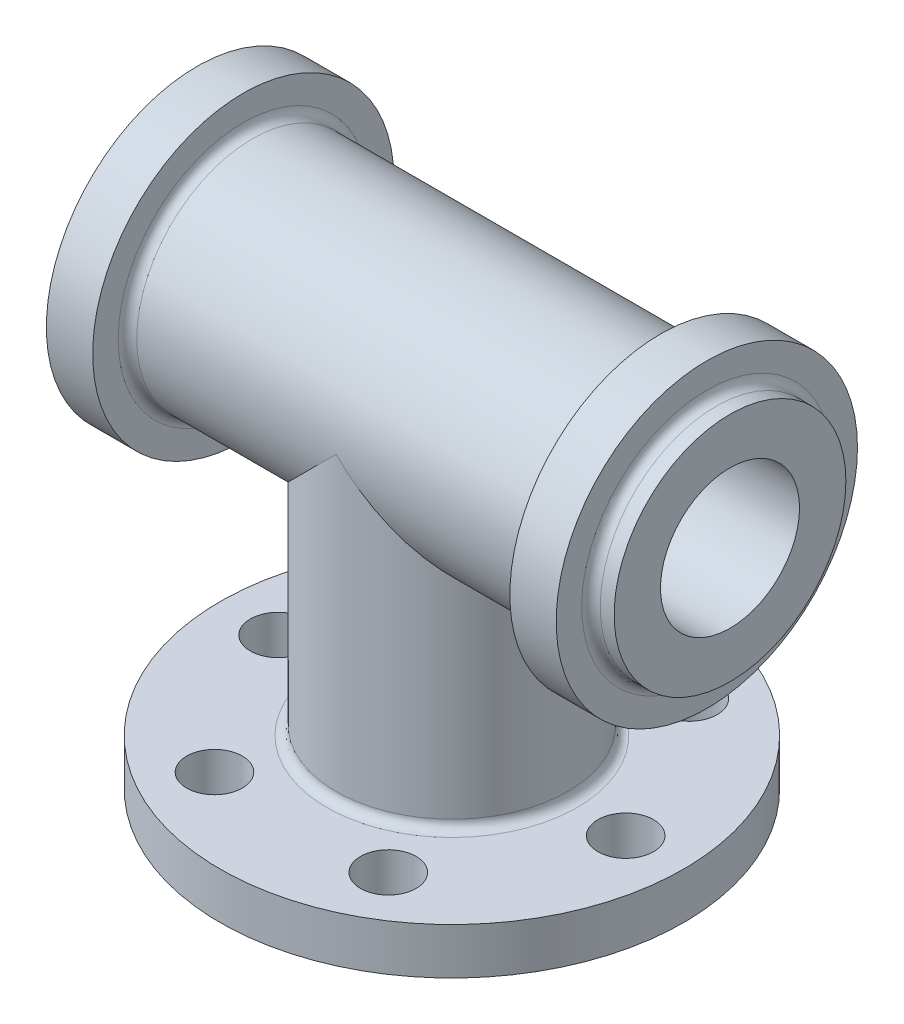
ISO-10303-21;
HEADER;
FILE_DESCRIPTION(('STEP AP214'),'2;1');
FILE_NAME('part.step','',(''),(''),'','','');
FILE_SCHEMA(('AUTOMOTIVE_DESIGN { 1 0 10303 214 1 1 1 1 }'));
ENDSEC;
DATA;
#1=APPLICATION_CONTEXT('core data for automotive mechanical design processes');
#2=APPLICATION_PROTOCOL_DEFINITION('international standard','automotive_design',2000,#1);
#3=PRODUCT_CONTEXT('',#1,'mechanical');
#4=PRODUCT('Part','Part','',(#3));
#5=PRODUCT_RELATED_PRODUCT_CATEGORY('part','',(#4));
#6=PRODUCT_DEFINITION_FORMATION('','',#4);
#7=PRODUCT_DEFINITION_CONTEXT('part definition',#1,'design');
#8=PRODUCT_DEFINITION('design','',#6,#7);
#9=PRODUCT_DEFINITION_SHAPE('','',#8);
#10=(LENGTH_UNIT() NAMED_UNIT(*) SI_UNIT(.MILLI.,.METRE.));
#11=(NAMED_UNIT(*) PLANE_ANGLE_UNIT() SI_UNIT($,.RADIAN.));
#12=(NAMED_UNIT(*) SI_UNIT($,.STERADIAN.) SOLID_ANGLE_UNIT());
#13=UNCERTAINTY_MEASURE_WITH_UNIT(LENGTH_MEASURE(1.E-05),#10,'distance_accuracy_value','');
#14=(GEOMETRIC_REPRESENTATION_CONTEXT(3) GLOBAL_UNCERTAINTY_ASSIGNED_CONTEXT((#13)) GLOBAL_UNIT_ASSIGNED_CONTEXT((#10,
#11,#12)) REPRESENTATION_CONTEXT('',''));
#15=CARTESIAN_POINT('',(0.,0.,0.));
#16=DIRECTION('',(0.,0.,1.));
#17=DIRECTION('',(1.,0.,0.));
#18=AXIS2_PLACEMENT_3D('',#15,#16,#17);
#19=CARTESIAN_POINT('',(0.,-80.,0.));
#20=DIRECTION('',(0.,1.,0.));
#21=DIRECTION('',(0.,0.,1.));
#22=AXIS2_PLACEMENT_3D('',#19,#20,#21);
#23=CYLINDRICAL_SURFACE('',#22,25.);
#24=CARTESIAN_POINT('',(0.,-63.,0.));
#25=DIRECTION('',(0.,-1.,0.));
#26=DIRECTION('',(0.,0.,-1.));
#27=AXIS2_PLACEMENT_3D('',#24,#25,#26);
#28=CIRCLE('',#27,25.);
#29=CARTESIAN_POINT('',(0.,-63.,-25.));
#30=VERTEX_POINT('',#29);
#31=EDGE_CURVE('E81',#30,#30,#28,.F.);
#32=ORIENTED_EDGE('',*,*,#31,.T.);
#33=EDGE_LOOP('',(#32));
#34=FACE_BOUND('',#33,.T.);
#35=CARTESIAN_POINT('',(0.,0.,0.));
#36=DIRECTION('',(-0.707106781186547,0.707106781186547,0.));
#37=DIRECTION('',(-0.707106781186547,-0.707106781186547,0.));
#38=AXIS2_PLACEMENT_3D('',#35,#36,#37);
#39=ELLIPSE('',#38,35.3553390593274,25.);
#40=CARTESIAN_POINT('',(0.,0.,-25.));
#41=VERTEX_POINT('',#40);
#42=CARTESIAN_POINT('',(0.,0.,25.));
#43=VERTEX_POINT('',#42);
#44=EDGE_CURVE('E65',#41,#43,#39,.T.);
#45=ORIENTED_EDGE('',*,*,#44,.F.);
#46=CARTESIAN_POINT('',(0.,0.,0.));
#47=DIRECTION('',(-0.707106781186547,-0.707106781186547,0.));
#48=DIRECTION('',(-0.707106781186547,0.707106781186547,0.));
#49=AXIS2_PLACEMENT_3D('',#46,#47,#48);
#50=ELLIPSE('',#49,35.3553390593274,25.);
#51=EDGE_CURVE('E182',#43,#41,#50,.F.);
#52=ORIENTED_EDGE('',*,*,#51,.F.);
#53=EDGE_LOOP('',(#45,#52));
#54=FACE_BOUND('',#53,.T.);
#55=ADVANCED_FACE('F41',(#34,#54),#23,.T.);
#56=CARTESIAN_POINT('',(60.,0.,0.));
#57=DIRECTION('',(-1.,0.,0.));
#58=DIRECTION('',(0.,0.,1.));
#59=AXIS2_PLACEMENT_3D('',#56,#57,#58);
#60=CYLINDRICAL_SURFACE('',#59,25.);
#61=CARTESIAN_POINT('',(43.,0.,0.));
#62=DIRECTION('',(1.,0.,0.));
#63=DIRECTION('',(0.,0.,-1.));
#64=AXIS2_PLACEMENT_3D('',#61,#62,#63);
#65=CIRCLE('',#64,25.);
#66=CARTESIAN_POINT('',(43.,0.,-25.));
#67=VERTEX_POINT('',#66);
#68=EDGE_CURVE('E98',#67,#67,#65,.F.);
#69=ORIENTED_EDGE('',*,*,#68,.T.);
#70=EDGE_LOOP('',(#69));
#71=FACE_BOUND('',#70,.T.);
#72=CARTESIAN_POINT('',(-43.,0.,0.));
#73=DIRECTION('',(-1.,0.,0.));
#74=DIRECTION('',(0.,0.,1.));
#75=AXIS2_PLACEMENT_3D('',#72,#73,#74);
#76=CIRCLE('',#75,25.);
#77=CARTESIAN_POINT('',(-43.,0.,25.));
#78=VERTEX_POINT('',#77);
#79=EDGE_CURVE('E92',#78,#78,#76,.F.);
#80=ORIENTED_EDGE('',*,*,#79,.T.);
#81=EDGE_LOOP('',(#80));
#82=FACE_BOUND('',#81,.T.);
#83=ORIENTED_EDGE('',*,*,#51,.T.);
#84=ORIENTED_EDGE('',*,*,#44,.T.);
#85=EDGE_LOOP('',(#83,#84));
#86=FACE_BOUND('',#85,.T.);
#87=ADVANCED_FACE('F127',(#71,#82,#86),#60,.T.);
#88=CARTESIAN_POINT('',(45.,0.,0.));
#89=DIRECTION('',(1.,0.,0.));
#90=DIRECTION('',(0.,0.,-1.));
#91=AXIS2_PLACEMENT_3D('',#88,#89,#90);
#92=CYLINDRICAL_SURFACE('',#91,32.5);
#93=CARTESIAN_POINT('',(45.,0.,0.));
#94=DIRECTION('',(1.,0.,0.));
#95=DIRECTION('',(0.,0.,-1.));
#96=AXIS2_PLACEMENT_3D('',#93,#94,#95);
#97=CIRCLE('',#96,32.5);
#98=CARTESIAN_POINT('',(45.,0.,-32.5));
#99=VERTEX_POINT('',#98);
#100=EDGE_CURVE('E174',#99,#99,#97,.T.);
#101=ORIENTED_EDGE('',*,*,#100,.T.);
#102=EDGE_LOOP('',(#101));
#103=FACE_BOUND('',#102,.T.);
#104=CARTESIAN_POINT('',(55.,0.,0.));
#105=DIRECTION('',(1.,0.,0.));
#106=DIRECTION('',(0.,0.,-1.));
#107=AXIS2_PLACEMENT_3D('',#104,#105,#106);
#108=CIRCLE('',#107,32.5);
#109=CARTESIAN_POINT('',(55.,0.,-32.5));
#110=VERTEX_POINT('',#109);
#111=EDGE_CURVE('E168',#110,#110,#108,.T.);
#112=ORIENTED_EDGE('',*,*,#111,.F.);
#113=EDGE_LOOP('',(#112));
#114=FACE_BOUND('',#113,.T.);
#115=ADVANCED_FACE('F131',(#103,#114),#92,.T.);
#116=CARTESIAN_POINT('',(45.,0.,0.));
#117=DIRECTION('',(1.,0.,0.));
#118=DIRECTION('',(0.,0.,-1.));
#119=AXIS2_PLACEMENT_3D('',#116,#117,#118);
#120=PLANE('',#119);
#121=CARTESIAN_POINT('',(45.,0.,0.));
#122=DIRECTION('',(1.,0.,0.));
#123=DIRECTION('',(0.,0.,-1.));
#124=AXIS2_PLACEMENT_3D('',#121,#122,#123);
#125=CIRCLE('',#124,27.);
#126=CARTESIAN_POINT('',(45.,0.,-27.));
#127=VERTEX_POINT('',#126);
#128=EDGE_CURVE('E95',#127,#127,#125,.T.);
#129=ORIENTED_EDGE('',*,*,#128,.T.);
#130=EDGE_LOOP('',(#129));
#131=FACE_BOUND('',#130,.T.);
#132=ORIENTED_EDGE('',*,*,#100,.F.);
#133=EDGE_LOOP('',(#132));
#134=FACE_BOUND('',#133,.T.);
#135=ADVANCED_FACE('F239',(#131,#134),#120,.F.);
#136=CARTESIAN_POINT('',(55.,0.,0.));
#137=DIRECTION('',(1.,0.,0.));
#138=DIRECTION('',(0.,0.,-1.));
#139=AXIS2_PLACEMENT_3D('',#136,#137,#138);
#140=PLANE('',#139);
#141=CARTESIAN_POINT('',(55.,0.,0.));
#142=DIRECTION('',(1.,0.,0.));
#143=DIRECTION('',(0.,0.,-1.));
#144=AXIS2_PLACEMENT_3D('',#141,#142,#143);
#145=CIRCLE('',#144,27.);
#146=CARTESIAN_POINT('',(55.,0.,-27.));
#147=VERTEX_POINT('',#146);
#148=EDGE_CURVE('E90',#147,#147,#145,.F.);
#149=ORIENTED_EDGE('',*,*,#148,.T.);
#150=EDGE_LOOP('',(#149));
#151=FACE_BOUND('',#150,.T.);
#152=ORIENTED_EDGE('',*,*,#111,.T.);
#153=EDGE_LOOP('',(#152));
#154=FACE_BOUND('',#153,.T.);
#155=ADVANCED_FACE('F244',(#151,#154),#140,.T.);
#156=CARTESIAN_POINT('',(60.,0.,0.));
#157=DIRECTION('',(1.,0.,0.));
#158=DIRECTION('',(0.,0.,-1.));
#159=AXIS2_PLACEMENT_3D('',#156,#157,#158);
#160=PLANE('',#159);
#161=CARTESIAN_POINT('',(60.,0.,0.));
#162=DIRECTION('',(1.,0.,0.));
#163=DIRECTION('',(0.,0.,-1.));
#164=AXIS2_PLACEMENT_3D('',#161,#162,#163);
#165=CIRCLE('',#164,15.);
#166=CARTESIAN_POINT('',(60.,0.,-15.));
#167=VERTEX_POINT('',#166);
#168=EDGE_CURVE('E164',#167,#167,#165,.T.);
#169=ORIENTED_EDGE('',*,*,#168,.F.);
#170=EDGE_LOOP('',(#169));
#171=FACE_BOUND('',#170,.T.);
#172=CARTESIAN_POINT('',(60.,0.,0.));
#173=DIRECTION('',(1.,0.,0.));
#174=DIRECTION('',(0.,0.,-1.));
#175=AXIS2_PLACEMENT_3D('',#172,#173,#174);
#176=CIRCLE('',#175,25.);
#177=CARTESIAN_POINT('',(60.,0.,-25.));
#178=VERTEX_POINT('',#177);
#179=EDGE_CURVE('E176',#178,#178,#176,.T.);
#180=ORIENTED_EDGE('',*,*,#179,.T.);
#181=EDGE_LOOP('',(#180));
#182=FACE_BOUND('',#181,.T.);
#183=ADVANCED_FACE('F199',(#171,#182),#160,.T.);
#184=CARTESIAN_POINT('',(57.,0.,0.));
#185=DIRECTION('',(1.,0.,0.));
#186=DIRECTION('',(0.,0.,-1.));
#187=AXIS2_PLACEMENT_3D('',#184,#185,#186);
#188=CIRCLE('',#187,25.);
#189=CARTESIAN_POINT('',(57.,0.,-25.));
#190=VERTEX_POINT('',#189);
#191=EDGE_CURVE('E88',#190,#190,#188,.T.);
#192=ORIENTED_EDGE('',*,*,#191,.T.);
#193=EDGE_LOOP('',(#192));
#194=FACE_BOUND('',#193,.T.);
#195=ORIENTED_EDGE('',*,*,#179,.F.);
#196=EDGE_LOOP('',(#195));
#197=FACE_BOUND('',#196,.T.);
#198=ADVANCED_FACE('F136',(#194,#197),#60,.T.);
#199=CARTESIAN_POINT('',(-45.,0.,0.));
#200=DIRECTION('',(-1.,0.,0.));
#201=DIRECTION('',(0.,0.,-1.));
#202=AXIS2_PLACEMENT_3D('',#199,#200,#201);
#203=PLANE('',#202);
#204=CARTESIAN_POINT('',(-45.,0.,0.));
#205=DIRECTION('',(-1.,0.,0.));
#206=DIRECTION('',(0.,0.,1.));
#207=AXIS2_PLACEMENT_3D('',#204,#205,#206);
#208=CIRCLE('',#207,27.);
#209=CARTESIAN_POINT('',(-45.,0.,27.));
#210=VERTEX_POINT('',#209);
#211=EDGE_CURVE('E101',#210,#210,#208,.T.);
#212=ORIENTED_EDGE('',*,*,#211,.T.);
#213=EDGE_LOOP('',(#212));
#214=FACE_BOUND('',#213,.T.);
#215=CARTESIAN_POINT('',(-45.,0.,0.));
#216=DIRECTION('',(1.,0.,0.));
#217=DIRECTION('',(0.,0.,-1.));
#218=AXIS2_PLACEMENT_3D('',#215,#216,#217);
#219=CIRCLE('',#218,32.5);
#220=CARTESIAN_POINT('',(-45.,0.,-32.5));
#221=VERTEX_POINT('',#220);
#222=EDGE_CURVE('E165',#221,#221,#219,.T.);
#223=ORIENTED_EDGE('',*,*,#222,.T.);
#224=EDGE_LOOP('',(#223));
#225=FACE_BOUND('',#224,.T.);
#226=ADVANCED_FACE('F204',(#214,#225),#203,.F.);
#227=CARTESIAN_POINT('',(-55.,0.,0.));
#228=DIRECTION('',(-1.,0.,0.));
#229=DIRECTION('',(0.,0.,-1.));
#230=AXIS2_PLACEMENT_3D('',#227,#228,#229);
#231=PLANE('',#230);
#232=CARTESIAN_POINT('',(-55.,0.,0.));
#233=DIRECTION('',(-1.,0.,0.));
#234=DIRECTION('',(0.,0.,1.));
#235=AXIS2_PLACEMENT_3D('',#232,#233,#234);
#236=CIRCLE('',#235,27.);
#237=CARTESIAN_POINT('',(-55.,0.,27.));
#238=VERTEX_POINT('',#237);
#239=EDGE_CURVE('E102',#238,#238,#236,.F.);
#240=ORIENTED_EDGE('',*,*,#239,.T.);
#241=EDGE_LOOP('',(#240));
#242=FACE_BOUND('',#241,.T.);
#243=CARTESIAN_POINT('',(-55.,0.,0.));
#244=DIRECTION('',(1.,0.,0.));
#245=DIRECTION('',(0.,0.,-1.));
#246=AXIS2_PLACEMENT_3D('',#243,#244,#245);
#247=CIRCLE('',#246,32.5);
#248=CARTESIAN_POINT('',(-55.,0.,-32.5));
#249=VERTEX_POINT('',#248);
#250=EDGE_CURVE('E158',#249,#249,#247,.T.);
#251=ORIENTED_EDGE('',*,*,#250,.F.);
#252=EDGE_LOOP('',(#251));
#253=FACE_BOUND('',#252,.T.);
#254=ADVANCED_FACE('F198',(#242,#253),#231,.T.);
#255=CARTESIAN_POINT('',(-45.,0.,0.));
#256=DIRECTION('',(-1.,0.,0.));
#257=DIRECTION('',(0.,0.,1.));
#258=AXIS2_PLACEMENT_3D('',#255,#256,#257);
#259=CYLINDRICAL_SURFACE('',#258,32.5);
#260=ORIENTED_EDGE('',*,*,#222,.F.);
#261=EDGE_LOOP('',(#260));
#262=FACE_BOUND('',#261,.T.);
#263=ORIENTED_EDGE('',*,*,#250,.T.);
#264=EDGE_LOOP('',(#263));
#265=FACE_BOUND('',#264,.T.);
#266=ADVANCED_FACE('F186',(#262,#265),#259,.T.);
#267=CARTESIAN_POINT('',(-60.,0.,0.));
#268=DIRECTION('',(1.,0.,0.));
#269=DIRECTION('',(0.,0.,-1.));
#270=AXIS2_PLACEMENT_3D('',#267,#268,#269);
#271=PLANE('',#270);
#272=CARTESIAN_POINT('',(-60.,0.,0.));
#273=DIRECTION('',(1.,0.,0.));
#274=DIRECTION('',(0.,0.,-1.));
#275=AXIS2_PLACEMENT_3D('',#272,#273,#274);
#276=CIRCLE('',#275,15.);
#277=CARTESIAN_POINT('',(-60.,0.,-15.));
#278=VERTEX_POINT('',#277);
#279=EDGE_CURVE('E157',#278,#278,#276,.T.);
#280=ORIENTED_EDGE('',*,*,#279,.T.);
#281=EDGE_LOOP('',(#280));
#282=FACE_BOUND('',#281,.T.);
#283=CARTESIAN_POINT('',(-60.,0.,0.));
#284=DIRECTION('',(1.,0.,0.));
#285=DIRECTION('',(0.,0.,-1.));
#286=AXIS2_PLACEMENT_3D('',#283,#284,#285);
#287=CIRCLE('',#286,25.);
#288=CARTESIAN_POINT('',(-60.,0.,-25.));
#289=VERTEX_POINT('',#288);
#290=EDGE_CURVE('E173',#289,#289,#287,.T.);
#291=ORIENTED_EDGE('',*,*,#290,.F.);
#292=EDGE_LOOP('',(#291));
#293=FACE_BOUND('',#292,.T.);
#294=ADVANCED_FACE('F151',(#282,#293),#271,.F.);
#295=CARTESIAN_POINT('',(-57.,0.,0.));
#296=DIRECTION('',(-1.,0.,0.));
#297=DIRECTION('',(0.,0.,1.));
#298=AXIS2_PLACEMENT_3D('',#295,#296,#297);
#299=CIRCLE('',#298,25.);
#300=CARTESIAN_POINT('',(-57.,0.,25.));
#301=VERTEX_POINT('',#300);
#302=EDGE_CURVE('E110',#301,#301,#299,.T.);
#303=ORIENTED_EDGE('',*,*,#302,.T.);
#304=EDGE_LOOP('',(#303));
#305=FACE_BOUND('',#304,.T.);
#306=ORIENTED_EDGE('',*,*,#290,.T.);
#307=EDGE_LOOP('',(#306));
#308=FACE_BOUND('',#307,.T.);
#309=ADVANCED_FACE('F140',(#305,#308),#60,.T.);
#310=CARTESIAN_POINT('',(0.,-75.,0.));
#311=DIRECTION('',(0.,-1.,0.));
#312=DIRECTION('',(0.,0.,-1.));
#313=AXIS2_PLACEMENT_3D('',#310,#311,#312);
#314=CIRCLE('',#313,25.);
#315=CARTESIAN_POINT('',(0.,-75.,-25.));
#316=VERTEX_POINT('',#315);
#317=EDGE_CURVE('E74',#316,#316,#314,.F.);
#318=ORIENTED_EDGE('',*,*,#317,.F.);
#319=EDGE_LOOP('',(#318));
#320=FACE_BOUND('',#319,.T.);
#321=CARTESIAN_POINT('',(0.,-80.,0.));
#322=DIRECTION('',(0.,1.,0.));
#323=DIRECTION('',(0.,0.,1.));
#324=AXIS2_PLACEMENT_3D('',#321,#322,#323);
#325=CIRCLE('',#324,25.);
#326=CARTESIAN_POINT('',(0.,-80.,25.));
#327=VERTEX_POINT('',#326);
#328=EDGE_CURVE('E160',#327,#327,#325,.T.);
#329=ORIENTED_EDGE('',*,*,#328,.T.);
#330=EDGE_LOOP('',(#329));
#331=FACE_BOUND('',#330,.T.);
#332=ADVANCED_FACE('F129',(#320,#331),#23,.T.);
#333=CARTESIAN_POINT('',(0.,-80.,0.));
#334=DIRECTION('',(0.,1.,0.));
#335=DIRECTION('',(0.,0.,1.));
#336=AXIS2_PLACEMENT_3D('',#333,#334,#335);
#337=CYLINDRICAL_SURFACE('',#336,15.);
#338=CARTESIAN_POINT('',(0.,-79.,0.));
#339=DIRECTION('',(0.,1.,0.));
#340=DIRECTION('',(0.,0.,1.));
#341=AXIS2_PLACEMENT_3D('',#338,#339,#340);
#342=CIRCLE('',#341,15.);
#343=CARTESIAN_POINT('',(0.,-79.,15.));
#344=VERTEX_POINT('',#343);
#345=EDGE_CURVE('E11',#344,#344,#342,.F.);
#346=ORIENTED_EDGE('',*,*,#345,.T.);
#347=EDGE_LOOP('',(#346));
#348=FACE_BOUND('',#347,.T.);
#349=CARTESIAN_POINT('',(0.,0.,0.));
#350=DIRECTION('',(0.707106781186547,-0.707106781186547,0.));
#351=DIRECTION('',(0.707106781186547,0.707106781186547,0.));
#352=AXIS2_PLACEMENT_3D('',#349,#350,#351);
#353=ELLIPSE('',#352,21.2132034355964,15.);
#354=CARTESIAN_POINT('',(0.,0.,15.));
#355=VERTEX_POINT('',#354);
#356=CARTESIAN_POINT('',(0.,0.,-15.));
#357=VERTEX_POINT('',#356);
#358=EDGE_CURVE('E66',#355,#357,#353,.T.);
#359=ORIENTED_EDGE('',*,*,#358,.F.);
#360=CARTESIAN_POINT('',(0.,0.,0.));
#361=DIRECTION('',(0.707106781186547,0.707106781186547,0.));
#362=DIRECTION('',(0.707106781186547,-0.707106781186547,0.));
#363=AXIS2_PLACEMENT_3D('',#360,#361,#362);
#364=ELLIPSE('',#363,21.2132034355964,15.);
#365=EDGE_CURVE('E57',#357,#355,#364,.F.);
#366=ORIENTED_EDGE('',*,*,#365,.F.);
#367=EDGE_LOOP('',(#359,#366));
#368=FACE_BOUND('',#367,.T.);
#369=ADVANCED_FACE('F69',(#348,#368),#337,.F.);
#370=CARTESIAN_POINT('',(0.,-80.,0.));
#371=DIRECTION('',(0.,1.,0.));
#372=DIRECTION('',(0.,0.,1.));
#373=AXIS2_PLACEMENT_3D('',#370,#371,#372);
#374=PLANE('',#373);
#375=CARTESIAN_POINT('',(0.,-80.,0.));
#376=DIRECTION('',(0.,1.,0.));
#377=DIRECTION('',(0.,0.,1.));
#378=AXIS2_PLACEMENT_3D('',#375,#376,#377);
#379=CIRCLE('',#378,16.);
#380=CARTESIAN_POINT('',(0.,-80.,16.));
#381=VERTEX_POINT('',#380);
#382=EDGE_CURVE('E49',#381,#381,#379,.T.);
#383=ORIENTED_EDGE('',*,*,#382,.T.);
#384=EDGE_LOOP('',(#383));
#385=FACE_BOUND('',#384,.T.);
#386=ORIENTED_EDGE('',*,*,#328,.F.);
#387=EDGE_LOOP('',(#386));
#388=FACE_BOUND('',#387,.T.);
#389=ADVANCED_FACE('F115',(#385,#388),#374,.F.);
#390=CARTESIAN_POINT('',(60.,0.,0.));
#391=DIRECTION('',(1.,0.,0.));
#392=DIRECTION('',(0.,0.,-1.));
#393=AXIS2_PLACEMENT_3D('',#390,#391,#392);
#394=CYLINDRICAL_SURFACE('',#393,15.);
#395=ORIENTED_EDGE('',*,*,#358,.T.);
#396=ORIENTED_EDGE('',*,*,#365,.T.);
#397=EDGE_LOOP('',(#395,#396));
#398=FACE_BOUND('',#397,.T.);
#399=ORIENTED_EDGE('',*,*,#279,.F.);
#400=EDGE_LOOP('',(#399));
#401=FACE_BOUND('',#400,.T.);
#402=ORIENTED_EDGE('',*,*,#168,.T.);
#403=EDGE_LOOP('',(#402));
#404=FACE_BOUND('',#403,.T.);
#405=ADVANCED_FACE('F75',(#398,#401,#404),#394,.F.);
#406=CARTESIAN_POINT('',(0.,-65.,0.));
#407=DIRECTION('',(0.,-1.,0.));
#408=DIRECTION('',(0.,0.,-1.));
#409=AXIS2_PLACEMENT_3D('',#406,#407,#408);
#410=CYLINDRICAL_SURFACE('',#409,50.);
#411=CARTESIAN_POINT('',(0.,-65.,0.));
#412=DIRECTION('',(0.,-1.,0.));
#413=DIRECTION('',(0.,0.,-1.));
#414=AXIS2_PLACEMENT_3D('',#411,#412,#413);
#415=CIRCLE('',#414,50.);
#416=CARTESIAN_POINT('',(0.,-65.,-50.));
#417=VERTEX_POINT('',#416);
#418=EDGE_CURVE('E467',#417,#417,#415,.T.);
#419=ORIENTED_EDGE('',*,*,#418,.T.);
#420=EDGE_LOOP('',(#419));
#421=FACE_BOUND('',#420,.T.);
#422=CARTESIAN_POINT('',(0.,-75.,0.));
#423=DIRECTION('',(0.,-1.,0.));
#424=DIRECTION('',(0.,0.,-1.));
#425=AXIS2_PLACEMENT_3D('',#422,#423,#424);
#426=CIRCLE('',#425,50.);
#427=CARTESIAN_POINT('',(0.,-75.,-50.));
#428=VERTEX_POINT('',#427);
#429=EDGE_CURVE('E470',#428,#428,#426,.T.);
#430=ORIENTED_EDGE('',*,*,#429,.F.);
#431=EDGE_LOOP('',(#430));
#432=FACE_BOUND('',#431,.T.);
#433=ADVANCED_FACE('F287',(#421,#432),#410,.T.);
#434=CARTESIAN_POINT('',(0.,-65.,0.));
#435=DIRECTION('',(0.,-1.,0.));
#436=DIRECTION('',(0.,0.,-1.));
#437=AXIS2_PLACEMENT_3D('',#434,#435,#436);
#438=PLANE('',#437);
#439=CARTESIAN_POINT('',(0.,-65.,0.));
#440=DIRECTION('',(0.,-1.,0.));
#441=DIRECTION('',(0.,0.,-1.));
#442=AXIS2_PLACEMENT_3D('',#439,#440,#441);
#443=CIRCLE('',#442,27.);
#444=CARTESIAN_POINT('',(0.,-65.,-27.));
#445=VERTEX_POINT('',#444);
#446=EDGE_CURVE('E79',#445,#445,#443,.T.);
#447=ORIENTED_EDGE('',*,*,#446,.T.);
#448=EDGE_LOOP('',(#447));
#449=FACE_BOUND('',#448,.T.);
#450=CARTESIAN_POINT('',(18.7500000000004,-65.,32.4759526419162));
#451=DIRECTION('',(0.,-1.,0.));
#452=DIRECTION('',(0.,0.,-1.));
#453=AXIS2_PLACEMENT_3D('',#450,#451,#452);
#454=CIRCLE('',#453,5.99999999999999);
#455=CARTESIAN_POINT('',(18.7500000000004,-65.,26.4759526419162));
#456=VERTEX_POINT('',#455);
#457=EDGE_CURVE('E435',#456,#456,#454,.T.);
#458=ORIENTED_EDGE('',*,*,#457,.T.);
#459=EDGE_LOOP('',(#458));
#460=FACE_BOUND('',#459,.T.);
#461=CARTESIAN_POINT('',(-18.7499999999997,-65.,32.4759526419166));
#462=DIRECTION('',(0.,-1.,0.));
#463=DIRECTION('',(0.,0.,-1.));
#464=AXIS2_PLACEMENT_3D('',#461,#462,#463);
#465=CIRCLE('',#464,5.99999999999999);
#466=CARTESIAN_POINT('',(-18.7499999999997,-65.,26.4759526419166));
#467=VERTEX_POINT('',#466);
#468=EDGE_CURVE('E439',#467,#467,#465,.T.);
#469=ORIENTED_EDGE('',*,*,#468,.T.);
#470=EDGE_LOOP('',(#469));
#471=FACE_BOUND('',#470,.T.);
#472=CARTESIAN_POINT('',(-37.5,-65.,2.61861100413235E-13));
#473=DIRECTION('',(0.,-1.,0.));
#474=DIRECTION('',(0.,0.,-1.));
#475=AXIS2_PLACEMENT_3D('',#472,#473,#474);
#476=CIRCLE('',#475,6.);
#477=CARTESIAN_POINT('',(-37.5,-65.,-5.99999999999973));
#478=VERTEX_POINT('',#477);
#479=EDGE_CURVE('E447',#478,#478,#476,.T.);
#480=ORIENTED_EDGE('',*,*,#479,.T.);
#481=EDGE_LOOP('',(#480));
#482=FACE_BOUND('',#481,.T.);
#483=CARTESIAN_POINT('',(-18.7500000000001,-65.,-32.4759526419164));
#484=DIRECTION('',(0.,-1.,0.));
#485=DIRECTION('',(0.,0.,-1.));
#486=AXIS2_PLACEMENT_3D('',#483,#484,#485);
#487=CIRCLE('',#486,6.);
#488=CARTESIAN_POINT('',(-18.7500000000001,-65.,-38.4759526419164));
#489=VERTEX_POINT('',#488);
#490=EDGE_CURVE('E455',#489,#489,#487,.T.);
#491=ORIENTED_EDGE('',*,*,#490,.T.);
#492=EDGE_LOOP('',(#491));
#493=FACE_BOUND('',#492,.T.);
#494=CARTESIAN_POINT('',(18.7499999999999,-65.,-32.4759526419165));
#495=DIRECTION('',(0.,-1.,0.));
#496=DIRECTION('',(0.,0.,-1.));
#497=AXIS2_PLACEMENT_3D('',#494,#495,#496);
#498=CIRCLE('',#497,6.);
#499=CARTESIAN_POINT('',(18.7499999999999,-65.,-38.4759526419165));
#500=VERTEX_POINT('',#499);
#501=EDGE_CURVE('E456',#500,#500,#498,.T.);
#502=ORIENTED_EDGE('',*,*,#501,.T.);
#503=EDGE_LOOP('',(#502));
#504=FACE_BOUND('',#503,.T.);
#505=CARTESIAN_POINT('',(37.5,-65.,0.));
#506=DIRECTION('',(0.,-1.,0.));
#507=DIRECTION('',(0.,0.,-1.));
#508=AXIS2_PLACEMENT_3D('',#505,#506,#507);
#509=CIRCLE('',#508,5.99999999999999);
#510=CARTESIAN_POINT('',(37.5,-65.,-5.99999999999999));
#511=VERTEX_POINT('',#510);
#512=EDGE_CURVE('E461',#511,#511,#509,.T.);
#513=ORIENTED_EDGE('',*,*,#512,.T.);
#514=EDGE_LOOP('',(#513));
#515=FACE_BOUND('',#514,.T.);
#516=ORIENTED_EDGE('',*,*,#418,.F.);
#517=EDGE_LOOP('',(#516));
#518=FACE_BOUND('',#517,.T.);
#519=ADVANCED_FACE('F288',(#449,#460,#471,#482,#493,#504,#515,#518),#438,.F.);
#520=CARTESIAN_POINT('',(0.,-75.,0.));
#521=DIRECTION('',(0.,-1.,0.));
#522=DIRECTION('',(0.,0.,-1.));
#523=AXIS2_PLACEMENT_3D('',#520,#521,#522);
#524=PLANE('',#523);
#525=CARTESIAN_POINT('',(18.7500000000004,-75.,32.4759526419162));
#526=DIRECTION('',(0.,-1.,0.));
#527=DIRECTION('',(0.,0.,-1.));
#528=AXIS2_PLACEMENT_3D('',#525,#526,#527);
#529=CIRCLE('',#528,5.99999999999999);
#530=CARTESIAN_POINT('',(18.7500000000004,-75.,26.4759526419162));
#531=VERTEX_POINT('',#530);
#532=EDGE_CURVE('E434',#531,#531,#529,.T.);
#533=ORIENTED_EDGE('',*,*,#532,.F.);
#534=EDGE_LOOP('',(#533));
#535=FACE_BOUND('',#534,.T.);
#536=CARTESIAN_POINT('',(-18.7499999999997,-75.,32.4759526419166));
#537=DIRECTION('',(0.,-1.,0.));
#538=DIRECTION('',(0.,0.,-1.));
#539=AXIS2_PLACEMENT_3D('',#536,#537,#538);
#540=CIRCLE('',#539,5.99999999999999);
#541=CARTESIAN_POINT('',(-18.7499999999997,-75.,26.4759526419166));
#542=VERTEX_POINT('',#541);
#543=EDGE_CURVE('E440',#542,#542,#540,.T.);
#544=ORIENTED_EDGE('',*,*,#543,.F.);
#545=EDGE_LOOP('',(#544));
#546=FACE_BOUND('',#545,.T.);
#547=CARTESIAN_POINT('',(-37.5,-75.,2.61861100413235E-13));
#548=DIRECTION('',(0.,-1.,0.));
#549=DIRECTION('',(0.,0.,-1.));
#550=AXIS2_PLACEMENT_3D('',#547,#548,#549);
#551=CIRCLE('',#550,6.);
#552=CARTESIAN_POINT('',(-37.5,-75.,-5.99999999999973));
#553=VERTEX_POINT('',#552);
#554=EDGE_CURVE('E444',#553,#553,#551,.T.);
#555=ORIENTED_EDGE('',*,*,#554,.F.);
#556=EDGE_LOOP('',(#555));
#557=FACE_BOUND('',#556,.T.);
#558=CARTESIAN_POINT('',(-18.7500000000001,-75.,-32.4759526419164));
#559=DIRECTION('',(0.,-1.,0.));
#560=DIRECTION('',(0.,0.,-1.));
#561=AXIS2_PLACEMENT_3D('',#558,#559,#560);
#562=CIRCLE('',#561,6.);
#563=CARTESIAN_POINT('',(-18.7500000000001,-75.,-38.4759526419164));
#564=VERTEX_POINT('',#563);
#565=EDGE_CURVE('E446',#564,#564,#562,.T.);
#566=ORIENTED_EDGE('',*,*,#565,.F.);
#567=EDGE_LOOP('',(#566));
#568=FACE_BOUND('',#567,.T.);
#569=CARTESIAN_POINT('',(18.7499999999999,-75.,-32.4759526419165));
#570=DIRECTION('',(0.,-1.,0.));
#571=DIRECTION('',(0.,0.,-1.));
#572=AXIS2_PLACEMENT_3D('',#569,#570,#571);
#573=CIRCLE('',#572,6.);
#574=CARTESIAN_POINT('',(18.7499999999999,-75.,-38.4759526419165));
#575=VERTEX_POINT('',#574);
#576=EDGE_CURVE('E452',#575,#575,#573,.T.);
#577=ORIENTED_EDGE('',*,*,#576,.F.);
#578=EDGE_LOOP('',(#577));
#579=FACE_BOUND('',#578,.T.);
#580=ORIENTED_EDGE('',*,*,#317,.T.);
#581=EDGE_LOOP('',(#580));
#582=FACE_BOUND('',#581,.T.);
#583=CARTESIAN_POINT('',(37.5,-75.,0.));
#584=DIRECTION('',(0.,-1.,0.));
#585=DIRECTION('',(0.,0.,-1.));
#586=AXIS2_PLACEMENT_3D('',#583,#584,#585);
#587=CIRCLE('',#586,5.99999999999999);
#588=CARTESIAN_POINT('',(37.5,-75.,-5.99999999999999));
#589=VERTEX_POINT('',#588);
#590=EDGE_CURVE('E462',#589,#589,#587,.T.);
#591=ORIENTED_EDGE('',*,*,#590,.F.);
#592=EDGE_LOOP('',(#591));
#593=FACE_BOUND('',#592,.T.);
#594=ORIENTED_EDGE('',*,*,#429,.T.);
#595=EDGE_LOOP('',(#594));
#596=FACE_BOUND('',#595,.T.);
#597=ADVANCED_FACE('F289',(#535,#546,#557,#568,#579,#582,#593,#596),#524,.T.);
#598=CARTESIAN_POINT('',(37.5,-65.,0.));
#599=DIRECTION('',(0.,-1.,0.));
#600=DIRECTION('',(0.,0.,-1.));
#601=AXIS2_PLACEMENT_3D('',#598,#599,#600);
#602=CYLINDRICAL_SURFACE('',#601,5.99999999999999);
#603=ORIENTED_EDGE('',*,*,#512,.F.);
#604=EDGE_LOOP('',(#603));
#605=FACE_BOUND('',#604,.T.);
#606=ORIENTED_EDGE('',*,*,#590,.T.);
#607=EDGE_LOOP('',(#606));
#608=FACE_BOUND('',#607,.T.);
#609=ADVANCED_FACE('F364',(#605,#608),#602,.F.);
#610=CARTESIAN_POINT('',(18.7499999999999,-65.,-32.4759526419165));
#611=DIRECTION('',(0.,-1.,0.));
#612=DIRECTION('',(0.,0.,-1.));
#613=AXIS2_PLACEMENT_3D('',#610,#611,#612);
#614=CYLINDRICAL_SURFACE('',#613,6.);
#615=ORIENTED_EDGE('',*,*,#501,.F.);
#616=EDGE_LOOP('',(#615));
#617=FACE_BOUND('',#616,.T.);
#618=ORIENTED_EDGE('',*,*,#576,.T.);
#619=EDGE_LOOP('',(#618));
#620=FACE_BOUND('',#619,.T.);
#621=ADVANCED_FACE('F372',(#617,#620),#614,.F.);
#622=CARTESIAN_POINT('',(-18.7500000000001,-65.,-32.4759526419164));
#623=DIRECTION('',(0.,-1.,0.));
#624=DIRECTION('',(0.,0.,-1.));
#625=AXIS2_PLACEMENT_3D('',#622,#623,#624);
#626=CYLINDRICAL_SURFACE('',#625,6.);
#627=ORIENTED_EDGE('',*,*,#490,.F.);
#628=EDGE_LOOP('',(#627));
#629=FACE_BOUND('',#628,.T.);
#630=ORIENTED_EDGE('',*,*,#565,.T.);
#631=EDGE_LOOP('',(#630));
#632=FACE_BOUND('',#631,.T.);
#633=ADVANCED_FACE('F382',(#629,#632),#626,.F.);
#634=CARTESIAN_POINT('',(-37.5,-65.,2.61861100413235E-13));
#635=DIRECTION('',(0.,-1.,0.));
#636=DIRECTION('',(0.,0.,-1.));
#637=AXIS2_PLACEMENT_3D('',#634,#635,#636);
#638=CYLINDRICAL_SURFACE('',#637,6.);
#639=ORIENTED_EDGE('',*,*,#479,.F.);
#640=EDGE_LOOP('',(#639));
#641=FACE_BOUND('',#640,.T.);
#642=ORIENTED_EDGE('',*,*,#554,.T.);
#643=EDGE_LOOP('',(#642));
#644=FACE_BOUND('',#643,.T.);
#645=ADVANCED_FACE('F394',(#641,#644),#638,.F.);
#646=CARTESIAN_POINT('',(-18.7499999999997,-65.,32.4759526419166));
#647=DIRECTION('',(0.,-1.,0.));
#648=DIRECTION('',(0.,0.,-1.));
#649=AXIS2_PLACEMENT_3D('',#646,#647,#648);
#650=CYLINDRICAL_SURFACE('',#649,5.99999999999999);
#651=ORIENTED_EDGE('',*,*,#468,.F.);
#652=EDGE_LOOP('',(#651));
#653=FACE_BOUND('',#652,.T.);
#654=ORIENTED_EDGE('',*,*,#543,.T.);
#655=EDGE_LOOP('',(#654));
#656=FACE_BOUND('',#655,.T.);
#657=ADVANCED_FACE('F402',(#653,#656),#650,.F.);
#658=CARTESIAN_POINT('',(18.7500000000004,-65.,32.4759526419162));
#659=DIRECTION('',(0.,-1.,0.));
#660=DIRECTION('',(0.,0.,-1.));
#661=AXIS2_PLACEMENT_3D('',#658,#659,#660);
#662=CYLINDRICAL_SURFACE('',#661,5.99999999999999);
#663=ORIENTED_EDGE('',*,*,#457,.F.);
#664=EDGE_LOOP('',(#663));
#665=FACE_BOUND('',#664,.T.);
#666=ORIENTED_EDGE('',*,*,#532,.T.);
#667=EDGE_LOOP('',(#666));
#668=FACE_BOUND('',#667,.T.);
#669=ADVANCED_FACE('F209',(#665,#668),#662,.F.);
#670=CARTESIAN_POINT('',(0.,-63.,0.));
#671=DIRECTION('',(0.,-1.,0.));
#672=DIRECTION('',(0.,0.,-1.));
#673=AXIS2_PLACEMENT_3D('',#670,#671,#672);
#674=TOROIDAL_SURFACE('',#673,27.,2.);
#675=ORIENTED_EDGE('',*,*,#31,.F.);
#676=EDGE_LOOP('',(#675));
#677=FACE_BOUND('',#676,.T.);
#678=ORIENTED_EDGE('',*,*,#446,.F.);
#679=EDGE_LOOP('',(#678));
#680=FACE_BOUND('',#679,.T.);
#681=ADVANCED_FACE('F206',(#677,#680),#674,.F.);
#682=CARTESIAN_POINT('',(57.,0.,0.));
#683=DIRECTION('',(1.,0.,0.));
#684=DIRECTION('',(0.,0.,-1.));
#685=AXIS2_PLACEMENT_3D('',#682,#683,#684);
#686=TOROIDAL_SURFACE('',#685,27.,2.);
#687=ORIENTED_EDGE('',*,*,#148,.F.);
#688=EDGE_LOOP('',(#687));
#689=FACE_BOUND('',#688,.T.);
#690=ORIENTED_EDGE('',*,*,#191,.F.);
#691=EDGE_LOOP('',(#690));
#692=FACE_BOUND('',#691,.T.);
#693=ADVANCED_FACE('F207',(#689,#692),#686,.F.);
#694=CARTESIAN_POINT('',(43.,0.,0.));
#695=DIRECTION('',(1.,0.,0.));
#696=DIRECTION('',(0.,0.,-1.));
#697=AXIS2_PLACEMENT_3D('',#694,#695,#696);
#698=TOROIDAL_SURFACE('',#697,27.,2.);
#699=ORIENTED_EDGE('',*,*,#68,.F.);
#700=EDGE_LOOP('',(#699));
#701=FACE_BOUND('',#700,.T.);
#702=ORIENTED_EDGE('',*,*,#128,.F.);
#703=EDGE_LOOP('',(#702));
#704=FACE_BOUND('',#703,.T.);
#705=ADVANCED_FACE('F212',(#701,#704),#698,.F.);
#706=CARTESIAN_POINT('',(-43.,0.,0.));
#707=DIRECTION('',(-1.,0.,0.));
#708=DIRECTION('',(0.,0.,1.));
#709=AXIS2_PLACEMENT_3D('',#706,#707,#708);
#710=TOROIDAL_SURFACE('',#709,27.,2.);
#711=ORIENTED_EDGE('',*,*,#79,.F.);
#712=EDGE_LOOP('',(#711));
#713=FACE_BOUND('',#712,.T.);
#714=ORIENTED_EDGE('',*,*,#211,.F.);
#715=EDGE_LOOP('',(#714));
#716=FACE_BOUND('',#715,.T.);
#717=ADVANCED_FACE('F125',(#713,#716),#710,.F.);
#718=CARTESIAN_POINT('',(-57.,0.,0.));
#719=DIRECTION('',(-1.,0.,0.));
#720=DIRECTION('',(0.,0.,1.));
#721=AXIS2_PLACEMENT_3D('',#718,#719,#720);
#722=TOROIDAL_SURFACE('',#721,27.,2.);
#723=ORIENTED_EDGE('',*,*,#302,.F.);
#724=EDGE_LOOP('',(#723));
#725=FACE_BOUND('',#724,.T.);
#726=ORIENTED_EDGE('',*,*,#239,.F.);
#727=EDGE_LOOP('',(#726));
#728=FACE_BOUND('',#727,.T.);
#729=ADVANCED_FACE('F117',(#725,#728),#722,.F.);
#730=CARTESIAN_POINT('',(0.,-80.,0.));
#731=DIRECTION('',(0.,-1.,0.));
#732=DIRECTION('',(0.,0.,-1.));
#733=AXIS2_PLACEMENT_3D('',#730,#731,#732);
#734=CONICAL_SURFACE('',#733,16.,0.785398163397441);
#735=ORIENTED_EDGE('',*,*,#345,.F.);
#736=EDGE_LOOP('',(#735));
#737=FACE_BOUND('',#736,.T.);
#738=ORIENTED_EDGE('',*,*,#382,.F.);
#739=EDGE_LOOP('',(#738));
#740=FACE_BOUND('',#739,.T.);
#741=ADVANCED_FACE('F42',(#737,#740),#734,.F.);
#742=CLOSED_SHELL('',(#55,#87,#115,#135,#155,#183,#198,#226,#254,#266,#294,#309,#332,#369,#389,
#405,#433,#519,#597,#609,#621,#633,#645,#657,#669,#681,#693,#705,#717,#729,#741));
#743=MANIFOLD_SOLID_BREP('B2',#742);
#744=ADVANCED_BREP_SHAPE_REPRESENTATION('',(#18,#743),#14);
#745=SHAPE_DEFINITION_REPRESENTATION(#9,#744);
ENDSEC;
END-ISO-10303-21;
